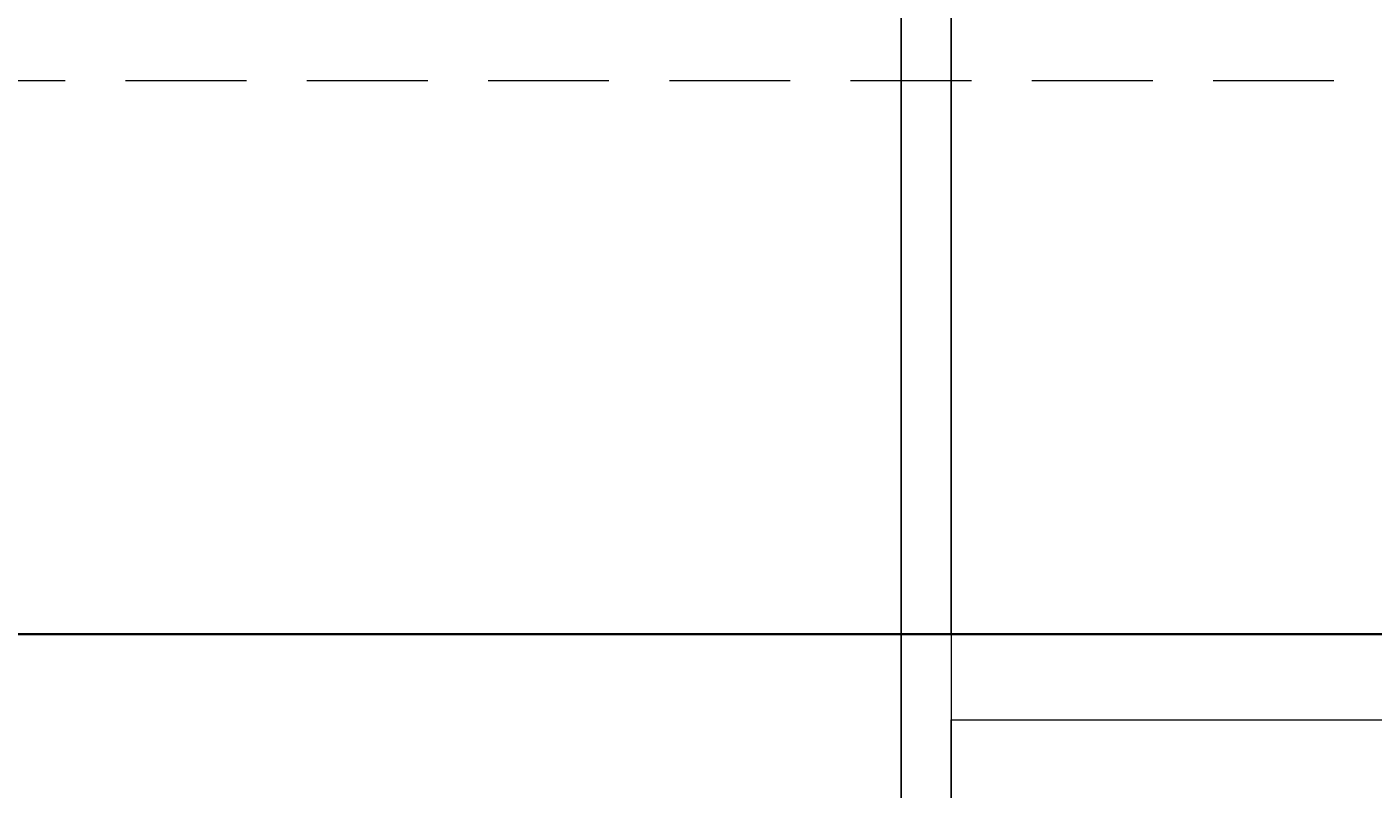
# Model space of a CAD drawing. Units: inches. Extents: x 1770 to 2988, y 1161 to 3221.
# Tile 17 of 44: x 2159 to 2229, y 2369 to 2409. Entities that reach past the tile are written whole.
import ezdxf

# ---------------------------------------------------------------- set-up
doc = ezdxf.new("R2010")
doc.units = ezdxf.units.IN
doc.linetypes.add('DASHED2', pattern=[9.525, 6.35, -3.175])
for name, color, linetype, lineweight in [('A-ANNO-DIMS', 2, 'Continuous', 18), ('A-GLAZ', 4, 'Continuous', 18), ('A-ROOF-OVHD', 7, 'DASHED2', 18), ('A-WALL', 7, 'Continuous', 35)]:
    doc.layers.add(name, color=color, linetype=linetype, lineweight=lineweight)
doc.styles.get("Standard").update_dxf_attribs({"font": 'arial.ttf'})
doc.dimstyles.get("Standard").update_dxf_attribs({"dimtxt": 0.18, "dimasz": 0.18, "dimexe": 0.18, "dimexo": 0.0625, "dimgap": 0.09, "dimtad": 0, "dimtih": 1, "dimtoh": 1, "dimdec": 4, "dimzin": 0, "dimdsep": 46, "dimtxsty": 'Standard', "dimcen": 0.09, "dimadec": 0, "dimazin": 0, "dimtfac": 1, "dimtdec": 4, "dimtofl": 0, "dimtmove": 0, "dimatfit": 3, "dimfxl": 1, "dimtolj": 1, "dimtzin": 0, "dimarcsym": 0})

# ---------------------------------------------------------------- blocks, each defined once
blk = doc.blocks.new('WIN-60-EXT')
for p, q in [((0, 9), (0, 0)), ((60, 4.5), (60, 9)), ((60, 9), (60, 0)), ((0, 0), (0, 4.5)), ((0, 4.5), (60, 4.5))]:
    blk.add_line(p, q)
blk = doc.blocks.new('*D64')
at = {"layer": 'A-ANNO-DIMS', "color": 0, "lineweight": -2, "transparency": 16777216}
for p, q in [((2151.696, 2376.765), (2151.696, 2570.705)), ((2151.876, 2570.525), (2179.093, 2570.525)), ((2207.098, 2570.525), (2179.881, 2570.525)), ((2207.278, 2376.765), (2207.278, 2570.705))]:
    blk.add_line(p, q, dxfattribs=at)
at = {"layer": 'A-ANNO-DIMS', "color": 0, "transparency": 16777216}
for points in [[(2151.876, 2570.555), (2151.876, 2570.495), (2151.696, 2570.525)], [(2207.098, 2570.555), (2207.098, 2570.495), (2207.278, 2570.525)]]:
    blk.add_solid(points, dxfattribs=at)
at = {"layer": 'Defpoints', "color": 0, "transparency": 16777216}
for p in [(2207.278, 2570.525), (2151.696, 2376.702), (2207.278, 2376.702)]:
    blk.add_point(p, dxfattribs=at)
at = {"layer": 'A-ANNO-DIMS', "color": 0, "transparency": 16777216, "insert": (2179.487, 2570.525), "char_height": 0.18, "attachment_point": 5}
blk.add_mtext('\\A1;55.58', dxfattribs=at)
blk = doc.blocks.new('*D79')
at = {"layer": 'A-ANNO-DIMS', "color": 0, "lineweight": -2, "transparency": 16777216}
for p, q in [((2151.696, 1610.265), (2151.696, 2570.705)), ((2151.876, 2570.525), (2177.783, 2570.525)), ((2204.477, 2570.525), (2178.57, 2570.525)), ((2204.657, 1610.265), (2204.657, 2570.705))]:
    blk.add_line(p, q, dxfattribs=at)
at = {"layer": 'A-ANNO-DIMS', "color": 0, "transparency": 16777216}
for points in [[(2151.876, 2570.555), (2151.876, 2570.495), (2151.696, 2570.525)], [(2204.477, 2570.555), (2204.477, 2570.495), (2204.657, 2570.525)]]:
    blk.add_solid(points, dxfattribs=at)
at = {"layer": 'Defpoints', "color": 0, "transparency": 16777216}
for p in [(2204.657, 2570.525), (2151.696, 1610.202), (2204.657, 1610.202)]:
    blk.add_point(p, dxfattribs=at)
at = {"layer": 'A-ANNO-DIMS', "color": 0, "transparency": 16777216, "insert": (2178.176, 2570.525), "char_height": 0.18, "attachment_point": 5}
blk.add_mtext('\\A1;52.96', dxfattribs=at)

msp = doc.modelspace()

# ---------------------------------------------------------------- linework, layer by layer
at = {"layer": 'A-ROOF-OVHD'}
msp.add_line((2656.0216, 2405.7876), (2096.7313, 2405.7876), dxfattribs=at)
at = {"layer": 'A-WALL'}
msp.add_line((2151.696, 2376.7021), (2625.696, 2376.7021), dxfattribs=at)

# ---------------------------------------------------------------- block references
at = {"layer": 'A-GLAZ'}
msp.add_blockref('WIN-60-EXT', (2207.2778, 2367.702), dxfattribs=at)

# ---------------------------------------------------------------- dimensions: what is measured, and where the dimension line sits
at = {"layer": 'A-ANNO-DIMS'}
for base, p1, p2, picture, middle in [((2207.2776, 2570.5247), (2151.696, 2376.7021), (2207.2776, 2376.7021), '*D64', (2179.4868, 2570.5247)), ((2204.6568, 2570.5247), (2151.696, 1610.2021), (2204.6568, 1610.2021), '*D79', (2178.1764, 2570.5247))]:
    dim = msp.add_linear_dim(base=base, p1=p1, p2=p2, dimstyle='Standard', override={"dimdec": 2, "dimlfac": 1, "dimrnd": 0, "dimzin": 0, "dimdsep": 46, "dimlunit": 2}, dxfattribs=at)
    dim.commit()
    dim.dimension.update_dxf_attribs({"geometry": picture, "text_midpoint": middle})

doc.saveas('drawing.dxf')
